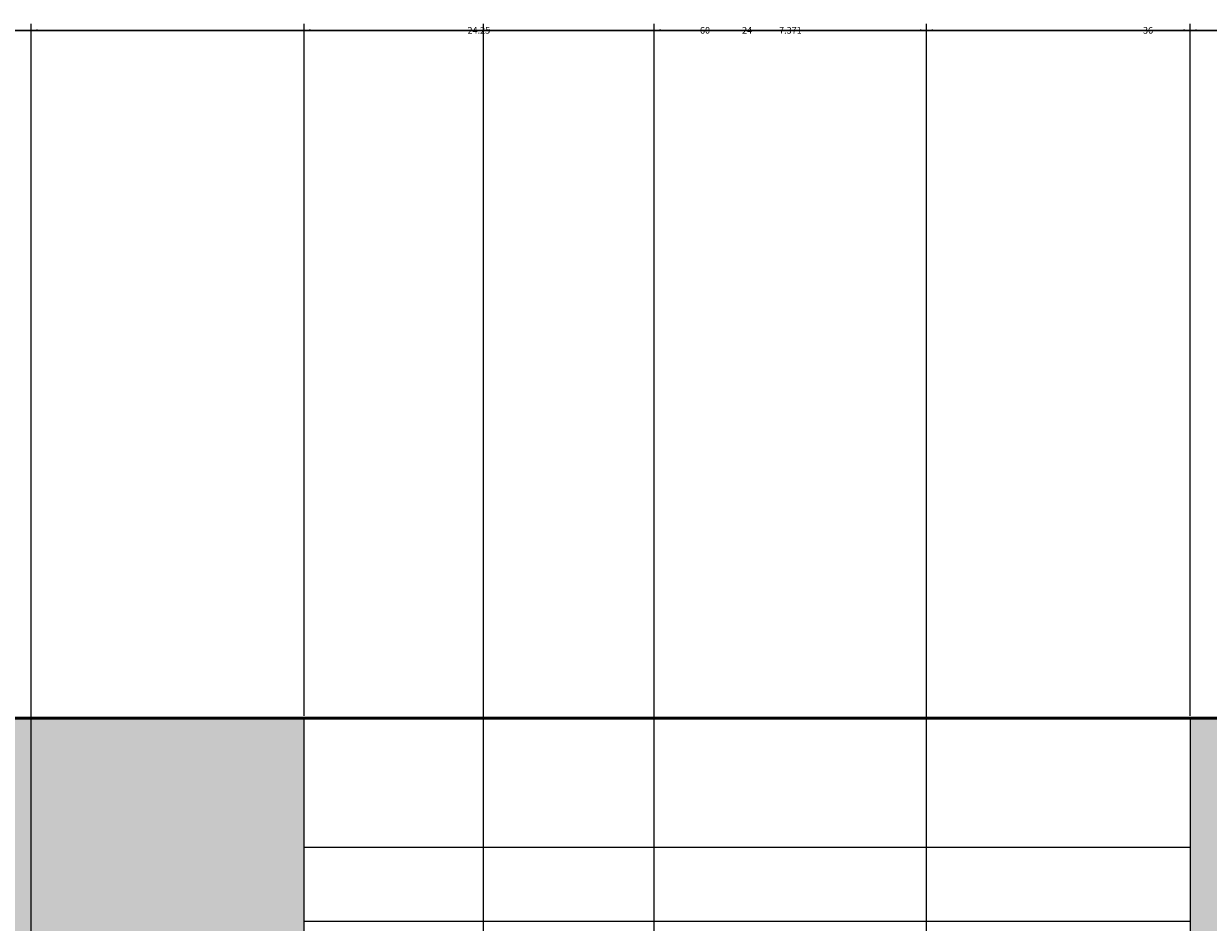
# Model space of a CAD drawing. Units: inches. Extents: x 2231 to 2461, y 2045 to 2455.
# Tile 93 of 95: x 2384 to 2416, y 2430 to 2455. Entities that reach past the tile are written whole.
import ezdxf

# ---------------------------------------------------------------- set-up
doc = ezdxf.new("R2010")
doc.units = ezdxf.units.IN
for name, color, linetype, lineweight in [('A-ANNO-DIMS', 2, 'Continuous', 18), ('A-GLAZ', 4, 'Continuous', 18), ('A-WALL', 7, 'Continuous', 50)]:
    doc.layers.add(name, color=color, linetype=linetype, lineweight=lineweight)
doc.layers.add('A-WALL-PATT', color=18, linetype='Continuous', lineweight=13, true_color=0x000000)
doc.styles.get("Standard").update_dxf_attribs({"font": 'arial.ttf'})
doc.dimstyles.get("Standard").update_dxf_attribs({"dimtxt": 0.18, "dimasz": 0.18, "dimexe": 0.18, "dimexo": 0.0625, "dimgap": 0.09, "dimtad": 0, "dimtih": 1, "dimtoh": 1, "dimdec": 4, "dimzin": 0, "dimdsep": 46, "dimtxsty": 'Standard', "dimcen": 0.09, "dimadec": 0, "dimazin": 0, "dimtfac": 1, "dimtdec": 4, "dimtofl": 0, "dimtmove": 0, "dimatfit": 3, "dimfxl": 1, "dimtolj": 1, "dimtzin": 0, "dimarcsym": 0})

# ---------------------------------------------------------------- blocks, each defined once
blk = doc.blocks.new('*D36')
at = {"layer": 'A-ANNO-DIMS', "color": 0, "lineweight": -2, "transparency": 16777216}
for p, q in [((2372.794, 2426.895), (2372.794, 2454.645)), ((2372.974, 2454.465), (2402.574, 2454.465)), ((2432.614, 2454.465), (2403.013, 2454.465)), ((2432.794, 2426.895), (2432.794, 2454.645))]:
    blk.add_line(p, q, dxfattribs=at)
at = {"layer": 'A-ANNO-DIMS', "color": 0, "transparency": 16777216}
for points in [[(2372.974, 2454.495), (2372.974, 2454.435), (2372.794, 2454.465)], [(2432.614, 2454.495), (2432.614, 2454.435), (2432.794, 2454.465)]]:
    blk.add_solid(points, dxfattribs=at)
at = {"layer": 'Defpoints', "color": 0, "transparency": 16777216}
for p in [(2432.794, 2454.465), (2372.794, 2426.833), (2432.794, 2426.833)]:
    blk.add_point(p, dxfattribs=at)
at = {"layer": 'A-ANNO-DIMS', "color": 0, "transparency": 16777216, "insert": (2402.794, 2454.465), "char_height": 0.18, "attachment_point": 5}
blk.add_mtext('\\A1;60', dxfattribs=at)
blk = doc.blocks.new('*D42')
at = {"layer": 'A-ANNO-DIMS', "color": 0, "lineweight": -2, "transparency": 16777216}
for p, q in [((2396.794, 2286.895), (2396.794, 2454.645)), ((2396.974, 2454.465), (2414.575, 2454.465)), ((2432.614, 2454.465), (2415.012, 2454.465)), ((2432.794, 2286.895), (2432.794, 2454.645))]:
    blk.add_line(p, q, dxfattribs=at)
at = {"layer": 'A-ANNO-DIMS', "color": 0, "transparency": 16777216}
for points in [[(2396.974, 2454.495), (2396.974, 2454.435), (2396.794, 2454.465)], [(2432.614, 2454.495), (2432.614, 2454.435), (2432.794, 2454.465)]]:
    blk.add_solid(points, dxfattribs=at)
at = {"layer": 'Defpoints', "color": 0, "transparency": 16777216}
for p in [(2432.794, 2454.465), (2396.794, 2286.833), (2432.794, 2286.833)]:
    blk.add_point(p, dxfattribs=at)
at = {"layer": 'A-ANNO-DIMS', "color": 0, "transparency": 16777216, "insert": (2414.794, 2454.465), "char_height": 0.18, "attachment_point": 5}
blk.add_mtext('\\A1;36', dxfattribs=at)
blk = doc.blocks.new('*D56')
at = {"layer": 'A-ANNO-DIMS', "color": 0, "lineweight": -2, "transparency": 16777216}
for p, q in [((2415.934, 2435.895), (2415.934, 2454.645)), ((2416.114, 2454.465), (2428.468, 2454.465)), ((2441.614, 2454.465), (2429.259, 2454.465)), ((2441.794, 2435.895), (2441.794, 2454.645))]:
    blk.add_line(p, q, dxfattribs=at)
at = {"layer": 'A-ANNO-DIMS', "color": 0, "transparency": 16777216}
for points in [[(2416.114, 2454.495), (2416.114, 2454.435), (2415.934, 2454.465)], [(2441.614, 2454.495), (2441.614, 2454.435), (2441.794, 2454.465)]]:
    blk.add_solid(points, dxfattribs=at)
at = {"layer": 'Defpoints', "color": 0, "transparency": 16777216}
for p in [(2441.794, 2454.465), (2415.934, 2435.833), (2441.794, 2435.833)]:
    blk.add_point(p, dxfattribs=at)
at = {"layer": 'A-ANNO-DIMS', "color": 0, "transparency": 16777216, "insert": (2428.864, 2454.465), "char_height": 0.18, "attachment_point": 5}
blk.add_mtext('\\A1;25.86', dxfattribs=at)
blk = doc.blocks.new('*D57')
at = {"layer": 'A-ANNO-DIMS', "color": 0, "lineweight": -2, "transparency": 16777216}
for p, q in [((2391.934, 2435.895), (2391.934, 2454.645)), ((2392.114, 2454.465), (2403.714, 2454.465)), ((2415.754, 2454.465), (2404.154, 2454.465)), ((2415.934, 2435.895), (2415.934, 2454.645))]:
    blk.add_line(p, q, dxfattribs=at)
at = {"layer": 'A-ANNO-DIMS', "color": 0, "transparency": 16777216}
for points in [[(2392.114, 2454.495), (2392.114, 2454.435), (2391.934, 2454.465)], [(2415.754, 2454.495), (2415.754, 2454.435), (2415.934, 2454.465)]]:
    blk.add_solid(points, dxfattribs=at)
at = {"layer": 'Defpoints', "color": 0, "transparency": 16777216}
for p in [(2415.934, 2454.465), (2391.934, 2435.833), (2415.934, 2435.833)]:
    blk.add_point(p, dxfattribs=at)
at = {"layer": 'A-ANNO-DIMS', "color": 0, "transparency": 16777216, "insert": (2403.934, 2454.465), "char_height": 0.18, "attachment_point": 5}
blk.add_mtext('\\A1;24', dxfattribs=at)
blk = doc.blocks.new('*D59')
at = {"layer": 'A-ANNO-DIMS', "color": 0, "lineweight": -2, "transparency": 16777216}
for p, q in [((2408.794, 2182.895), (2408.794, 2454.645)), ((2408.974, 2454.465), (2420.573, 2454.465)), ((2432.614, 2454.465), (2421.014, 2454.465)), ((2432.794, 2182.895), (2432.794, 2454.645))]:
    blk.add_line(p, q, dxfattribs=at)
at = {"layer": 'A-ANNO-DIMS', "color": 0, "transparency": 16777216}
for points in [[(2408.974, 2454.495), (2408.974, 2454.435), (2408.794, 2454.465)], [(2432.614, 2454.495), (2432.614, 2454.435), (2432.794, 2454.465)]]:
    blk.add_solid(points, dxfattribs=at)
at = {"layer": 'Defpoints', "color": 0, "transparency": 16777216}
for p in [(2432.794, 2454.465), (2408.794, 2182.833), (2432.794, 2182.833)]:
    blk.add_point(p, dxfattribs=at)
at = {"layer": 'A-ANNO-DIMS', "color": 0, "transparency": 16777216, "insert": (2420.794, 2454.465), "char_height": 0.18, "attachment_point": 5}
blk.add_mtext('\\A1;24', dxfattribs=at)
blk = doc.blocks.new('*D66')
at = {"layer": 'A-ANNO-DIMS', "color": 0, "lineweight": -2, "transparency": 16777216}
for p, q in [((2348.189, 2096.895), (2348.189, 2454.645)), ((2348.369, 2454.465), (2378.167, 2454.465)), ((2408.614, 2454.465), (2378.815, 2454.465)), ((2408.794, 2096.895), (2408.794, 2454.645))]:
    blk.add_line(p, q, dxfattribs=at)
at = {"layer": 'A-ANNO-DIMS', "color": 0, "transparency": 16777216}
for points in [[(2348.369, 2454.495), (2348.369, 2454.435), (2348.189, 2454.465)], [(2408.614, 2454.495), (2408.614, 2454.435), (2408.794, 2454.465)]]:
    blk.add_solid(points, dxfattribs=at)
at = {"layer": 'Defpoints', "color": 0, "transparency": 16777216}
for p in [(2408.794, 2454.465), (2348.189, 2096.833), (2408.794, 2096.833)]:
    blk.add_point(p, dxfattribs=at)
at = {"layer": 'A-ANNO-DIMS', "color": 0, "transparency": 16777216, "insert": (2378.491, 2454.465), "char_height": 0.18, "attachment_point": 5}
blk.add_mtext('\\A1;60.6', dxfattribs=at)
blk = doc.blocks.new('*D71')
at = {"layer": 'A-ANNO-DIMS', "color": 0, "lineweight": -2, "transparency": 16777216}
for p, q in [((2401.422, 2092.979), (2401.422, 2454.645)), ((2401.602, 2454.465), (2404.732, 2454.465)), ((2408.614, 2454.465), (2405.483, 2454.465)), ((2408.794, 2096.895), (2408.794, 2454.645))]:
    blk.add_line(p, q, dxfattribs=at)
at = {"layer": 'A-ANNO-DIMS', "color": 0, "transparency": 16777216}
for points in [[(2401.602, 2454.495), (2401.602, 2454.435), (2401.422, 2454.465)], [(2408.614, 2454.495), (2408.614, 2454.435), (2408.794, 2454.465)]]:
    blk.add_solid(points, dxfattribs=at)
at = {"layer": 'Defpoints', "color": 0, "transparency": 16777216}
for p in [(2408.794, 2454.465), (2408.794, 2096.833), (2401.422, 2092.917)]:
    blk.add_point(p, dxfattribs=at)
at = {"layer": 'A-ANNO-DIMS', "color": 0, "transparency": 16777216, "insert": (2405.108, 2454.465), "char_height": 0.18, "attachment_point": 5}
blk.add_mtext('\\A1;7.371', dxfattribs=at)
blk = doc.blocks.new('*D72')
at = {"layer": 'A-ANNO-DIMS', "color": 0, "lineweight": -2, "transparency": 16777216}
for p, q in [((2384.543, 2145.12), (2384.543, 2454.645)), ((2384.723, 2454.465), (2396.272, 2454.465)), ((2408.614, 2454.465), (2397.064, 2454.465)), ((2408.794, 2150.677), (2408.794, 2454.645))]:
    blk.add_line(p, q, dxfattribs=at)
at = {"layer": 'A-ANNO-DIMS', "color": 0, "transparency": 16777216}
for points in [[(2384.723, 2454.495), (2384.723, 2454.435), (2384.543, 2454.465)], [(2408.614, 2454.495), (2408.614, 2454.435), (2408.794, 2454.465)]]:
    blk.add_solid(points, dxfattribs=at)
at = {"layer": 'Defpoints', "color": 0, "transparency": 16777216}
for p in [(2408.794, 2454.465), (2408.794, 2150.615), (2384.543, 2145.058)]:
    blk.add_point(p, dxfattribs=at)
at = {"layer": 'A-ANNO-DIMS', "color": 0, "transparency": 16777216, "insert": (2396.668, 2454.465), "char_height": 0.18, "attachment_point": 5}
blk.add_mtext('\\A1;24.25', dxfattribs=at)

msp = doc.modelspace()

# ---------------------------------------------------------------- hatches: boundary and pattern name
at = {"layer": 'A-WALL-PATT'}
h = msp.add_hatch(color=256, dxfattribs=at)
h.dxf.hatch_style = 1
h.paths.add_polyline_path([(2441.7935, 2269.1535), (2432.7935, 2269.1535), (2432.7935, 2186.8328), (2396.7935, 2186.8328), (2396.7935, 2286.8328), (2394.7935, 2286.8328), (2394.7935, 2186.8328), (2334.7935, 2186.8328), (2334.7935, 2182.8328), (2432.7935, 2182.8328), (2432.7935, 2072.8328), (2416.6639, 2072.8328), (2416.6639, 2063.8328), (2441.7935, 2063.8328)])
h.paths.add_polyline_path([(2368.6639, 2072.8328), (2367.04, 2072.8328), (2330.7942, 2072.8328), (2330.7397, 2063.8328), (2368.6639, 2063.8328)])
h.paths.add_polyline_path([(2300.7392, 2068.3328), (2300.7392, 2072.8328), (2298.7935, 2072.8328), (2294.7935, 2072.8328), (2258.7935, 2072.8328), (2258.7935, 2120.8328), (2294.7935, 2120.8328), (2298.7935, 2120.8328), (2298.7935, 2128.8328), (2294.7935, 2128.8328), (2294.7935, 2124.8328), (2258.7935, 2124.8328), (2258.7935, 2182.8328), (2294.7935, 2182.8328), (2294.7935, 2174.8328), (2298.7935, 2174.8328), (2298.7935, 2182.8328), (2304.7935, 2182.8328), (2304.7935, 2186.8328), (2258.7935, 2186.8328), (2258.7935, 2221.999), (2249.7935, 2221.999), (2249.7935, 2063.8328), (2300.7392, 2063.8328)])
h.paths.add_polyline_path([(2391.9338, 2435.8328), (2333.82, 2435.8328), (2333.82, 2426.8328), (2368.7935, 2426.8328), (2368.7935, 2374.9508), (2368.7935, 2370.8328), (2372.3935, 2370.8328), (2372.7935, 2370.8328), (2372.7935, 2426.8328), (2391.9338, 2426.8328)])
h.paths.add_polyline_path([(2441.7935, 2435.8328), (2415.9338, 2435.8328), (2415.9338, 2426.8328), (2432.7935, 2426.8328), (2432.7935, 2334.8328), (2372.7935, 2334.8328), (2372.7935, 2346.8328), (2368.7935, 2346.8328), (2368.7935, 2306.8328), (2360.7935, 2306.8328), (2360.7935, 2302.8328), (2368.7935, 2302.8328), (2372.7935, 2302.8328), (2372.7935, 2330.8328), (2432.7935, 2330.8328), (2432.7935, 2317.1535), (2441.7935, 2317.1535)])
h.paths.add_polyline_path([(2285.82, 2435.8328), (2249.7935, 2435.8328), (2249.7935, 2269.999), (2258.7935, 2269.999), (2258.7935, 2302.8328), (2318.8168, 2302.8328), (2330.7935, 2302.8328), (2330.7935, 2306.8328), (2258.7935, 2306.8328), (2258.7935, 2426.8328), (2285.82, 2426.8328)])

# ---------------------------------------------------------------- linework, layer by layer
at = {"layer": 'A-GLAZ'}
for p, q in [((2391.9338, 2426.8328), (2391.9338, 2435.8328)), ((2415.9338, 2435.8328), (2415.9338, 2426.8328)), ((2391.9338, 2432.3328), (2415.9338, 2432.3328)), ((2391.9338, 2430.3328), (2415.9338, 2430.3328))]:
    msp.add_line(p, q, dxfattribs=at)
at = {"layer": 'A-WALL'}
msp.add_lwpolyline([(2300.7392, 2063.8328), (2249.7935, 2063.8328), (2249.7935, 2435.8328), (2441.7935, 2435.8328), (2441.7935, 2063.8328), (2330.7397, 2063.8328)], dxfattribs=at)

# ---------------------------------------------------------------- dimensions: what is measured, and where the dimension line sits
at = {"layer": 'A-ANNO-DIMS'}
for base, p1, p2, override, picture, middle in [((2408.7935, 2454.4653), (2348.1888, 2096.8328), (2408.7935, 2096.8328), {"dimdec": 1, "dimlfac": 1, "dimrnd": 0, "dimzin": 0, "dimdsep": 46, "dimlunit": 2}, '*D66', (2378.4912, 2454.4653)), ((2432.7935, 2454.4653), (2372.7935, 2426.8328), (2432.7935, 2426.8328), {"dimdec": 0, "dimlfac": 1, "dimrnd": 0, "dimzin": 0, "dimdsep": 46, "dimlunit": 2}, '*D36', (2402.7935, 2454.4653)), ((2408.7935, 2454.4653), (2384.5428, 2145.0576), (2408.7935, 2150.6145), {"dimdec": 2, "dimlfac": 1, "dimrnd": 0, "dimzin": 0, "dimdsep": 46, "dimlunit": 2}, '*D72', (2396.6682, 2454.4653)), ((2415.9338, 2454.4653), (2391.9338, 2435.8328), (2415.9338, 2435.8328), {"dimdec": 0, "dimlfac": 1, "dimrnd": 0, "dimzin": 0, "dimdsep": 46, "dimlunit": 2}, '*D57', (2403.9338, 2454.4653)), ((2432.7935, 2454.4653), (2396.7935, 2286.8328), (2432.7935, 2286.8328), {"dimdec": 0, "dimlfac": 1, "dimrnd": 0, "dimzin": 0, "dimdsep": 46, "dimlunit": 2}, '*D42', (2414.7935, 2454.4653)), ((2408.7935, 2454.4653), (2401.4221, 2092.9167), (2408.7935, 2096.8328), {"dimdec": 3, "dimlfac": 1, "dimrnd": 0, "dimzin": 0, "dimdsep": 46, "dimlunit": 2}, '*D71', (2405.1078, 2454.4653)), ((2432.7935, 2454.4653), (2408.7935, 2182.8328), (2432.7935, 2182.8328), {"dimdec": 0, "dimlfac": 1, "dimrnd": 0, "dimzin": 0, "dimdsep": 46, "dimlunit": 2}, '*D59', (2420.7935, 2454.4653)), ((2441.7935, 2454.4653), (2415.9338, 2435.8328), (2441.7935, 2435.8328), {"dimdec": 2, "dimlfac": 1, "dimrnd": 0, "dimzin": 0, "dimdsep": 46, "dimlunit": 2}, '*D56', (2428.8637, 2454.4653))]:
    dim = msp.add_linear_dim(base=base, p1=p1, p2=p2, dimstyle='Standard', override=override, dxfattribs=at)
    dim.commit()
    dim.dimension.update_dxf_attribs({"geometry": picture, "text_midpoint": middle})

doc.saveas('drawing.dxf')
